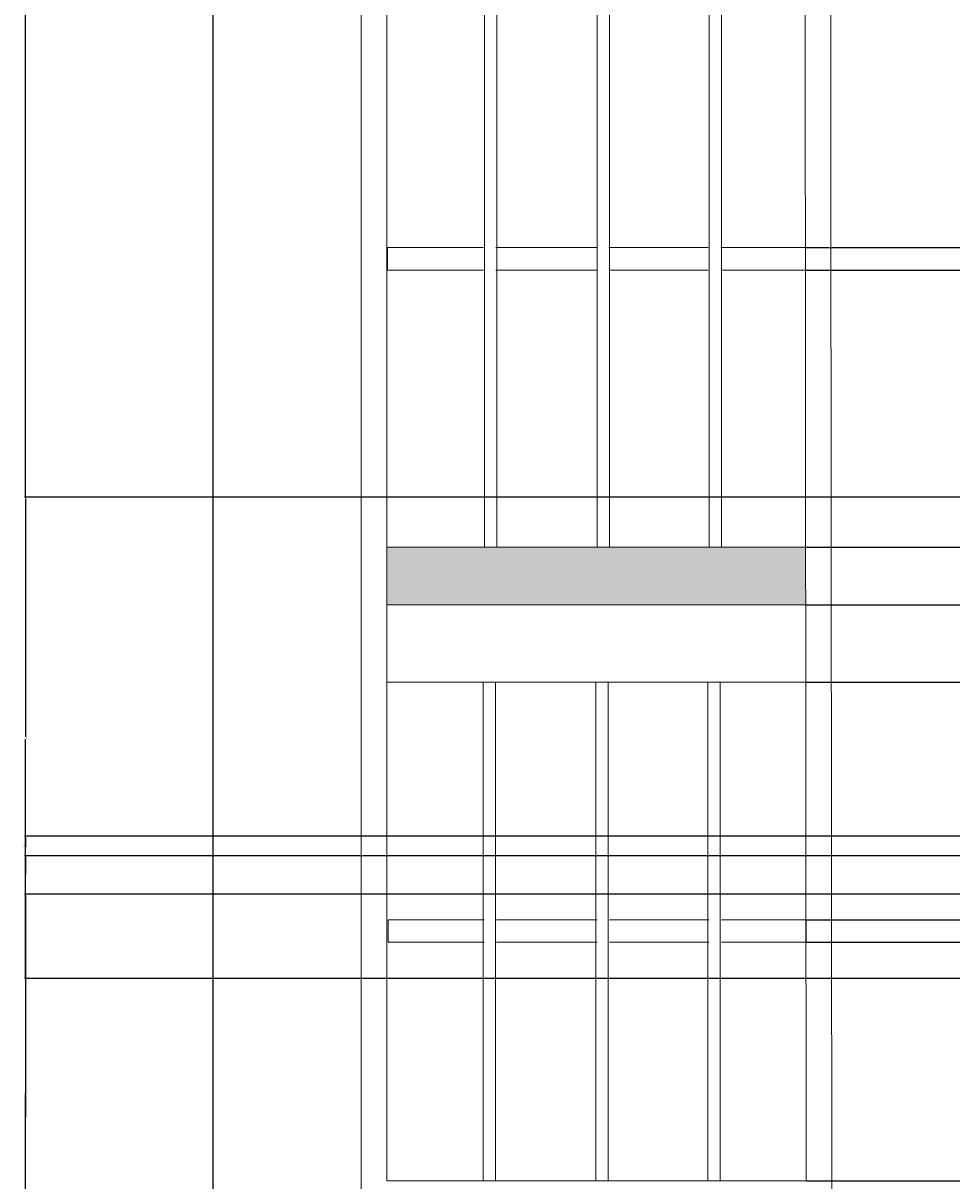
# Model space of a CAD drawing. Units: inches. Extents: x -14 to 375, y -86 to 549.
# Tile 6 of 12: x -14 to 130, y 156 to 336. Entities that reach past the tile are written whole.
import ezdxf

# ---------------------------------------------------------------- set-up
doc = ezdxf.new("R2010")
doc.units = ezdxf.units.IN
doc.header["$MEASUREMENT"] = 0
for name, color, linetype, lineweight in [('A-ANNO-DIMS', 2, 'Continuous', 18), ('A-ELEV', 7, 'Continuous', 25), ('A-ELEV-PATT', 8, 'Continuous', 13), ('A-GLAZ', 4, 'Continuous', 18)]:
    doc.layers.add(name, color=color, linetype=linetype, lineweight=lineweight)
doc.styles.get("Standard").update_dxf_attribs({"font": 'arial.ttf'})
doc.dimstyles.get("Standard").update_dxf_attribs({"dimtxt": 0.18, "dimasz": 0.18, "dimexe": 0.18, "dimexo": 0.0625, "dimgap": 0.09, "dimtad": 0, "dimtih": 1, "dimtoh": 1, "dimdec": 4, "dimzin": 0, "dimdsep": 46, "dimtxsty": 'Standard', "dimcen": 0.09, "dimadec": 0, "dimazin": 0, "dimtfac": 1, "dimtdec": 4, "dimtofl": 0, "dimtmove": 0, "dimatfit": 3, "dimfxl": 1, "dimtolj": 1, "dimtzin": 0, "dimarcsym": 0})

# ---------------------------------------------------------------- blocks, each defined once
blk = doc.blocks.new('*D15')
at = {"layer": 'A-ANNO-DIMS', "color": 0, "lineweight": -2, "transparency": 16777216}
for p, q in [((134.17, 187.85), (-13.88, 187.85)), ((-13.7, 187.67), (-13.7, 170.29)), ((-13.7, 152.56), (-13.7, 169.93)), ((38.44, 152.38), (-13.88, 152.38))]:
    blk.add_line(p, q, dxfattribs=at)
at = {"layer": 'A-ANNO-DIMS', "color": 0, "transparency": 16777216}
for points in [[(-13.73, 187.67), (-13.67, 187.67), (-13.7, 187.85)], [(-13.73, 152.56), (-13.67, 152.56), (-13.7, 152.38)]]:
    blk.add_solid(points, dxfattribs=at)
at = {"layer": 'Defpoints', "color": 0, "transparency": 16777216}
for p in [(-13.7, 187.85), (134.23, 187.85), (38.5, 152.38)]:
    blk.add_point(p, dxfattribs=at)
at = {"layer": 'A-ANNO-DIMS', "color": 0, "transparency": 16777216, "insert": (-13.7, 170.11), "char_height": 0.18, "attachment_point": 5}
blk.add_mtext('\\A1;35.47', dxfattribs=at)
blk = doc.blocks.new('*D16')
at = {"layer": 'A-ANNO-DIMS', "color": 0, "lineweight": -2, "transparency": 16777216}
for p, q in [((134.17, 262.71), (-13.88, 262.71)), ((-13.7, 262.53), (-13.7, 225.46)), ((-13.7, 188.03), (-13.7, 225.09)), ((134.17, 187.85), (-13.88, 187.85))]:
    blk.add_line(p, q, dxfattribs=at)
at = {"layer": 'A-ANNO-DIMS', "color": 0, "transparency": 16777216}
for points in [[(-13.73, 262.53), (-13.67, 262.53), (-13.7, 262.71)], [(-13.73, 188.03), (-13.67, 188.03), (-13.7, 187.85)]]:
    blk.add_solid(points, dxfattribs=at)
at = {"layer": 'Defpoints', "color": 0, "transparency": 16777216}
for p in [(-13.7, 262.71), (134.23, 262.71), (134.23, 187.85)]:
    blk.add_point(p, dxfattribs=at)
at = {"layer": 'A-ANNO-DIMS', "color": 0, "transparency": 16777216, "insert": (-13.7, 225.28), "char_height": 0.18, "attachment_point": 5}
blk.add_mtext('\\A1;74.86', dxfattribs=at)
blk = doc.blocks.new('*D17')
at = {"layer": 'A-ANNO-DIMS', "color": 0, "lineweight": -2, "transparency": 16777216}
for p, q in [((38.44, 432.97), (-13.88, 432.97)), ((-13.7, 432.79), (-13.7, 348.02)), ((-13.7, 262.89), (-13.7, 347.66)), ((134.17, 262.71), (-13.88, 262.71))]:
    blk.add_line(p, q, dxfattribs=at)
at = {"layer": 'A-ANNO-DIMS', "color": 0, "transparency": 16777216}
for points in [[(-13.73, 432.79), (-13.67, 432.79), (-13.7, 432.97)], [(-13.73, 262.89), (-13.67, 262.89), (-13.7, 262.71)]]:
    blk.add_solid(points, dxfattribs=at)
at = {"layer": 'Defpoints', "color": 0, "transparency": 16777216}
for p in [(-13.7, 432.97), (38.5, 432.97), (134.23, 262.71)]:
    blk.add_point(p, dxfattribs=at)
at = {"layer": 'A-ANNO-DIMS', "color": 0, "transparency": 16777216, "insert": (-13.7, 347.84), "char_height": 0.18, "attachment_point": 5}
blk.add_mtext('\\A1;170.26', dxfattribs=at)
blk = doc.blocks.new('*D29')
at = {"layer": 'A-ANNO-DIMS', "color": 0, "lineweight": -2, "transparency": 16777216}
for p, q in [((107.74, 193.48), (374.54, 193.48)), ((374.36, 193.3), (374.36, 175.11)), ((374.36, 156.56), (374.36, 174.75)), ((107.76, 156.38), (374.54, 156.38))]:
    blk.add_line(p, q, dxfattribs=at)
at = {"layer": 'A-ANNO-DIMS', "color": 0, "transparency": 16777216}
for points in [[(374.33, 193.3), (374.39, 193.3), (374.36, 193.48)], [(374.33, 156.56), (374.39, 156.56), (374.36, 156.38)]]:
    blk.add_solid(points, dxfattribs=at)
at = {"layer": 'Defpoints', "color": 0, "transparency": 16777216}
for p in [(107.68, 193.48), (374.36, 193.48), (107.7, 156.38)]:
    blk.add_point(p, dxfattribs=at)
at = {"layer": 'A-ANNO-DIMS', "color": 0, "transparency": 16777216, "insert": (374.36, 174.93), "char_height": 0.18, "attachment_point": 5}
blk.add_mtext('\\A1;37.106', dxfattribs=at)
blk = doc.blocks.new('*D30')
at = {"layer": 'A-ANNO-DIMS', "color": 0, "lineweight": -2, "transparency": 16777216}
for p, q in [((107.74, 196.98), (374.54, 196.98)), ((374.36, 196.8), (374.36, 195.41)), ((374.36, 193.66), (374.36, 195.05)), ((107.74, 193.48), (374.54, 193.48))]:
    blk.add_line(p, q, dxfattribs=at)
at = {"layer": 'A-ANNO-DIMS', "color": 0, "transparency": 16777216}
for points in [[(374.33, 196.8), (374.39, 196.8), (374.36, 196.98)], [(374.33, 193.66), (374.39, 193.66), (374.36, 193.48)]]:
    blk.add_solid(points, dxfattribs=at)
at = {"layer": 'Defpoints', "color": 0, "transparency": 16777216}
for p in [(107.68, 196.98), (374.36, 196.98), (107.68, 193.48)]:
    blk.add_point(p, dxfattribs=at)
at = {"layer": 'A-ANNO-DIMS', "color": 0, "transparency": 16777216, "insert": (374.36, 195.23), "char_height": 0.18, "attachment_point": 5}
blk.add_mtext('\\A1;3.501', dxfattribs=at)
blk = doc.blocks.new('*D31')
at = {"layer": 'A-ANNO-DIMS', "color": 0, "lineweight": -2, "transparency": 16777216}
for p, q in [((107.76, 233.96), (374.54, 233.96)), ((374.36, 233.78), (374.36, 215.65)), ((374.36, 197.16), (374.36, 215.29)), ((107.74, 196.98), (374.54, 196.98))]:
    blk.add_line(p, q, dxfattribs=at)
at = {"layer": 'A-ANNO-DIMS', "color": 0, "transparency": 16777216}
for points in [[(374.33, 233.78), (374.39, 233.78), (374.36, 233.96)], [(374.33, 197.16), (374.39, 197.16), (374.36, 196.98)]]:
    blk.add_solid(points, dxfattribs=at)
at = {"layer": 'Defpoints', "color": 0, "transparency": 16777216}
for p in [(107.7, 233.96), (374.36, 233.96), (107.68, 196.98)]:
    blk.add_point(p, dxfattribs=at)
at = {"layer": 'A-ANNO-DIMS', "color": 0, "transparency": 16777216, "insert": (374.36, 215.47), "char_height": 0.18, "attachment_point": 5}
blk.add_mtext('\\A1;36.975', dxfattribs=at)
blk = doc.blocks.new('*D32')
at = {"layer": 'A-ANNO-DIMS', "color": 0, "lineweight": -2, "transparency": 16777216}
for p, q in [((107.76, 245.96), (374.54, 245.96)), ((374.36, 245.78), (374.36, 240.14)), ((374.36, 234.14), (374.36, 239.78)), ((107.76, 233.96), (374.54, 233.96))]:
    blk.add_line(p, q, dxfattribs=at)
at = {"layer": 'A-ANNO-DIMS', "color": 0, "transparency": 16777216}
for points in [[(374.33, 245.78), (374.39, 245.78), (374.36, 245.96)], [(374.33, 234.14), (374.39, 234.14), (374.36, 233.96)]]:
    blk.add_solid(points, dxfattribs=at)
at = {"layer": 'Defpoints', "color": 0, "transparency": 16777216}
for p in [(107.7, 245.96), (374.36, 245.96), (107.7, 233.96)]:
    blk.add_point(p, dxfattribs=at)
at = {"layer": 'A-ANNO-DIMS', "color": 0, "transparency": 16777216, "insert": (374.36, 239.96), "char_height": 0.18, "attachment_point": 5}
blk.add_mtext('\\A1;12', dxfattribs=at)
blk = doc.blocks.new('*D33')
at = {"layer": 'A-ANNO-DIMS', "color": 0, "lineweight": -2, "transparency": 16777216}
for p, q in [((107.76, 254.96), (374.54, 254.96)), ((374.36, 254.78), (374.36, 250.64)), ((374.36, 246.14), (374.36, 250.28)), ((107.76, 245.96), (374.54, 245.96))]:
    blk.add_line(p, q, dxfattribs=at)
at = {"layer": 'A-ANNO-DIMS', "color": 0, "transparency": 16777216}
for points in [[(374.33, 254.78), (374.39, 254.78), (374.36, 254.96)], [(374.33, 246.14), (374.39, 246.14), (374.36, 245.96)]]:
    blk.add_solid(points, dxfattribs=at)
at = {"layer": 'Defpoints', "color": 0, "transparency": 16777216}
for p in [(107.7, 254.96), (374.36, 254.96), (107.7, 245.96)]:
    blk.add_point(p, dxfattribs=at)
at = {"layer": 'A-ANNO-DIMS', "color": 0, "transparency": 16777216, "insert": (374.36, 250.46), "char_height": 0.18, "attachment_point": 5}
blk.add_mtext('\\A1;9', dxfattribs=at)
blk = doc.blocks.new('*D34')
at = {"layer": 'A-ANNO-DIMS', "color": 0, "lineweight": -2, "transparency": 16777216}
for p, q in [((107.64, 298.04), (374.54, 298.04)), ((374.36, 297.86), (374.36, 276.68)), ((374.36, 255.14), (374.36, 276.32)), ((107.76, 254.96), (374.54, 254.96))]:
    blk.add_line(p, q, dxfattribs=at)
at = {"layer": 'A-ANNO-DIMS', "color": 0, "transparency": 16777216}
for points in [[(374.33, 297.86), (374.39, 297.86), (374.36, 298.04)], [(374.33, 255.14), (374.39, 255.14), (374.36, 254.96)]]:
    blk.add_solid(points, dxfattribs=at)
at = {"layer": 'Defpoints', "color": 0, "transparency": 16777216}
for p in [(107.58, 298.04), (374.36, 298.04), (107.7, 254.96)]:
    blk.add_point(p, dxfattribs=at)
at = {"layer": 'A-ANNO-DIMS', "color": 0, "transparency": 16777216, "insert": (374.36, 276.5), "char_height": 0.18, "attachment_point": 5}
blk.add_mtext('\\A1;43.08', dxfattribs=at)
blk = doc.blocks.new('*D35')
at = {"layer": 'A-ANNO-DIMS', "color": 0, "lineweight": -2, "transparency": 16777216}
for p, q in [((107.64, 301.54), (374.54, 301.54)), ((374.36, 301.36), (374.36, 299.97)), ((374.36, 298.22), (374.36, 299.6)), ((107.64, 298.04), (374.54, 298.04))]:
    blk.add_line(p, q, dxfattribs=at)
at = {"layer": 'A-ANNO-DIMS', "color": 0, "transparency": 16777216}
for points in [[(374.33, 301.36), (374.39, 301.36), (374.36, 301.54)], [(374.33, 298.22), (374.39, 298.22), (374.36, 298.04)]]:
    blk.add_solid(points, dxfattribs=at)
at = {"layer": 'Defpoints', "color": 0, "transparency": 16777216}
for p in [(107.58, 301.54), (374.36, 301.54), (107.58, 298.04)]:
    blk.add_point(p, dxfattribs=at)
at = {"layer": 'A-ANNO-DIMS', "color": 0, "transparency": 16777216, "insert": (374.36, 299.79), "char_height": 0.18, "attachment_point": 5}
blk.add_mtext('\\A1;3.501', dxfattribs=at)
blk = doc.blocks.new('*D36')
at = {"layer": 'A-ANNO-DIMS', "color": 0, "lineweight": -2, "transparency": 16777216}
for p, q in [((107.56, 353.96), (374.54, 353.96)), ((374.36, 353.78), (374.36, 327.93)), ((374.36, 301.72), (374.36, 327.57)), ((107.64, 301.54), (374.54, 301.54))]:
    blk.add_line(p, q, dxfattribs=at)
at = {"layer": 'A-ANNO-DIMS', "color": 0, "transparency": 16777216}
for points in [[(374.33, 353.78), (374.39, 353.78), (374.36, 353.96)], [(374.33, 301.72), (374.39, 301.72), (374.36, 301.54)]]:
    blk.add_solid(points, dxfattribs=at)
at = {"layer": 'Defpoints', "color": 0, "transparency": 16777216}
for p in [(107.5, 353.96), (374.36, 353.96), (107.58, 301.54)]:
    blk.add_point(p, dxfattribs=at)
at = {"layer": 'A-ANNO-DIMS', "color": 0, "transparency": 16777216, "insert": (374.36, 327.75), "char_height": 0.18, "attachment_point": 5}
blk.add_mtext('\\A1;52.42', dxfattribs=at)
blk = doc.blocks.new('*D96')
at = {"layer": 'A-ANNO-DIMS', "color": 0, "lineweight": -2, "transparency": 16777216}
for p, q in [((194.3, 200.95), (-13.88, 200.95)), ((-13.7, 200.77), (-13.7, 166.64)), ((-13.7, 132.15), (-13.7, 166.28)), ((194.3, 131.97), (-13.88, 131.97))]:
    blk.add_line(p, q, dxfattribs=at)
at = {"layer": 'A-ANNO-DIMS', "color": 0, "transparency": 16777216}
for points in [[(-13.73, 200.77), (-13.67, 200.77), (-13.7, 200.95)], [(-13.73, 132.15), (-13.67, 132.15), (-13.7, 131.97)]]:
    blk.add_solid(points, dxfattribs=at)
at = {"layer": 'Defpoints', "color": 0, "transparency": 16777216}
for p in [(-13.7, 200.95), (194.37, 200.95), (194.37, 131.97)]:
    blk.add_point(p, dxfattribs=at)
at = {"layer": 'A-ANNO-DIMS', "color": 0, "transparency": 16777216, "insert": (-13.7, 166.46), "char_height": 0.18, "attachment_point": 5}
blk.add_mtext('\\A1;68.98', dxfattribs=at)
blk = doc.blocks.new('*D97')
at = {"layer": 'A-ANNO-DIMS', "color": 0, "lineweight": -2, "transparency": 16777216}
for p, q in [((190.3, 206.95), (-13.88, 206.95)), ((-13.7, 206.77), (-13.7, 204.13)), ((-13.7, 201.13), (-13.7, 203.77)), ((194.3, 200.95), (-13.88, 200.95))]:
    blk.add_line(p, q, dxfattribs=at)
at = {"layer": 'A-ANNO-DIMS', "color": 0, "transparency": 16777216}
for points in [[(-13.73, 206.77), (-13.67, 206.77), (-13.7, 206.95)], [(-13.73, 201.13), (-13.67, 201.13), (-13.7, 200.95)]]:
    blk.add_solid(points, dxfattribs=at)
at = {"layer": 'Defpoints', "color": 0, "transparency": 16777216}
for p in [(-13.7, 206.95), (190.37, 206.95), (194.37, 200.95)]:
    blk.add_point(p, dxfattribs=at)
at = {"layer": 'A-ANNO-DIMS', "color": 0, "transparency": 16777216, "insert": (-13.7, 203.95), "char_height": 0.18, "attachment_point": 5}
blk.add_mtext('\\A1;6', dxfattribs=at)
blk = doc.blocks.new('*D98')
at = {"layer": 'A-ANNO-DIMS', "color": 0, "lineweight": -2, "transparency": 16777216}
for p, q in [((187.3, 209.97), (-13.88, 209.97)), ((-13.7, 209.79), (-13.7, 208.64)), ((-13.7, 207.13), (-13.7, 208.28)), ((190.3, 206.95), (-13.88, 206.95))]:
    blk.add_line(p, q, dxfattribs=at)
at = {"layer": 'A-ANNO-DIMS', "color": 0, "transparency": 16777216}
for points in [[(-13.73, 209.79), (-13.67, 209.79), (-13.7, 209.97)], [(-13.73, 207.13), (-13.67, 207.13), (-13.7, 206.95)]]:
    blk.add_solid(points, dxfattribs=at)
at = {"layer": 'Defpoints', "color": 0, "transparency": 16777216}
for p in [(-13.7, 209.97), (187.37, 209.97), (190.37, 206.95)]:
    blk.add_point(p, dxfattribs=at)
at = {"layer": 'A-ANNO-DIMS', "color": 0, "transparency": 16777216, "insert": (-13.7, 208.46), "char_height": 0.18, "attachment_point": 5}
blk.add_mtext('\\A1;3.023', dxfattribs=at)

msp = doc.modelspace()

# ---------------------------------------------------------------- hatches: boundary and pattern name
at = {"layer": 'A-ELEV-PATT'}
h = msp.add_hatch(dxfattribs=at)
h.set_pattern_fill('SWAMP', color=256, scale=0.8)
h.set_pattern_definition([(0, (-168.40604, -22.7026), (0.4, 0.6928203), [0.1, -0.7]), (90, (-168.35604, -22.7026), (-0.4, 0.69282032), [0.05, -1.3356406]), (90, (-168.34354, -22.7026), (-0.4, 0.69282032), [0.04, -1.3456406]), (90, (-168.36854, -22.7026), (-0.4, 0.69282032), [0.04, -1.3456406]), (60, (-168.33104, -22.7026), (-0.4, 0.6928203), [0.032, -0.768]), (120, (-168.38104, -22.7026), (-0.8, 3e-10), [0.032, -0.768])])
h.paths.add_polyline_path([(42.5033, 374.9589), (42.5033, 365.9589), (107.4987, 365.9589), (107.4987, 374.9589)])
h.paths.add_polyline_path([(107.615, 245.9589), (107.6063, 254.9589), (42.5033, 254.9589), (42.5033, 245.9589)])

# ---------------------------------------------------------------- linework, layer by layer
at = {"layer": 'A-ELEV'}
for p, q in [((15.4018, 365.9589), (15.4018, 245.9589)), ((15.4018, 245.9589), (15.4018, 125.9589))]:
    msp.add_line(p, q, dxfattribs=at)
at = {"layer": 'A-GLAZ'}
for p, q in [((107.4899, 374.9589), (107.7019, 156.3768)), ((57.6445, 254.9589), (57.6445, 353.9589)), ((59.5668, 353.9589), (59.5668, 254.9589)), ((75.2042, 254.9589), (75.2042, 353.9589)), ((77.1265, 353.9589), (77.1265, 254.9589)), ((92.5999, 254.9589), (92.5999, 353.9589)), ((94.5222, 353.9589), (94.5222, 254.9589)), ((42.5033, 254.9589), (107.7019, 254.9589)), ((59.5668, 254.9589), (57.6445, 254.9589)), ((77.1265, 254.9589), (75.2042, 254.9589)), ((94.5222, 254.9589), (92.5999, 254.9589)), ((42.5033, 245.9589), (107.7019, 245.9589)), ((107.7019, 245.9589), (42.5033, 245.9589)), ((42.5033, 233.9589), (107.7019, 233.9589)), ((107.7019, 156.3768), (42.5033, 156.3768))]:
    msp.add_line(p, q, dxfattribs=at)
for points in [[(111.4987, 365.9589), (111.7019, 152.3768), (38.5033, 152.3768), (38.5033, 365.9589), (38.5033, 432.9679, -0.90920588), (111.4987, 432.9679), (111.4987, 365.9589)], [(42.5033, 156.3768), (42.5033, 365.9589), (42.5033, 432.7722, -0.9040533), (107.4987, 432.7722), (107.4987, 365.9589)]]:
    msp.add_lwpolyline(points, format="xyb", dxfattribs=at)
for points in [[(57.521, 301.5363), (42.5831, 301.5363), (42.5831, 298.0352), (57.521, 298.0352)], [(75.0807, 301.5363), (59.4433, 301.5363)], [(92.4765, 301.5363), (77.003, 301.5363)], [(94.3987, 298.0352), (107.5784, 298.0352), (107.5784, 301.5363), (94.3987, 301.5363)], [(59.4433, 298.0352), (75.0807, 298.0352)], [(77.003, 298.0352), (92.4765, 298.0352)], [(59.3636, 233.9589), (59.3636, 156.3768), (57.4413, 156.3768), (57.4413, 233.9589)], [(76.9233, 233.9589), (76.9233, 156.3768), (75.001, 156.3768), (75.001, 233.9589)], [(94.319, 233.9589), (94.319, 156.3768), (92.3967, 156.3768), (92.3967, 233.9589)], [(57.6224, 196.9836), (42.6844, 196.9836), (42.6844, 193.4825), (57.6224, 193.4825)], [(75.1821, 196.9836), (59.5447, 196.9836)], [(92.5778, 196.9836), (77.1044, 196.9836)], [(94.5001, 193.4825), (107.6798, 193.4825), (107.6798, 196.9836), (94.5001, 196.9836)], [(59.5447, 193.4825), (75.1821, 193.4825)], [(77.1044, 193.4825), (92.5778, 193.4825)]]:
    msp.add_lwpolyline(points, dxfattribs=at)

# ---------------------------------------------------------------- dimensions: what is measured, and where the dimension line sits
at = {"layer": 'A-ANNO-DIMS'}
for base, p1, p2, override, picture, middle in [((-13.6982, 432.9679), (134.2334, 262.7071), (38.5033, 432.9679), {"dimdec": 2, "dimlfac": 1, "dimrnd": 0, "dimzin": 0, "dimdsep": 46, "dimlunit": 2}, '*D17', (-13.6982, 347.8375)), ((374.3647, 353.9589), (107.5784, 301.5363), (107.4987, 353.9589), {"dimdec": 2, "dimlfac": 1, "dimrnd": 0, "dimzin": 0, "dimdsep": 46, "dimlunit": 2}, '*D36', (374.3647, 327.7476)), ((374.3647, 301.5363), (107.5784, 298.0352), (107.5784, 301.5363), {"dimdec": 3, "dimlfac": 1, "dimrnd": 0, "dimzin": 0, "dimdsep": 46, "dimlunit": 2}, '*D35', (374.3647, 299.7857)), ((374.3647, 298.0352), (107.7019, 254.9589), (107.5784, 298.0352), {"dimdec": 2, "dimlfac": 1, "dimrnd": 0, "dimzin": 0, "dimdsep": 46, "dimlunit": 2}, '*D34', (374.3647, 276.4971)), ((-13.6982, 262.7071), (134.2334, 187.8466), (134.2334, 262.7071), {"dimdec": 2, "dimlfac": 1, "dimrnd": 0, "dimzin": 0, "dimdsep": 46, "dimlunit": 2}, '*D16', (-13.6982, 225.2768)), ((374.3647, 254.9589), (107.7019, 245.9589), (107.7019, 254.9589), {"dimdec": 0, "dimlfac": 1, "dimrnd": 0, "dimzin": 0, "dimdsep": 46, "dimlunit": 2}, '*D33', (374.3647, 250.4589)), ((374.3647, 245.9589), (107.7019, 233.9589), (107.7019, 245.9589), {"dimdec": 0, "dimlfac": 1, "dimrnd": 0, "dimzin": 0, "dimdsep": 46, "dimlunit": 2}, '*D32', (374.3647, 239.9589)), ((374.3647, 233.9589), (107.6798, 196.9836), (107.7019, 233.9589), {"dimdec": 3, "dimlfac": 1, "dimrnd": 0, "dimzin": 0, "dimdsep": 46, "dimlunit": 2}, '*D31', (374.3647, 215.4712)), ((-13.6982, 209.9717), (190.3657, 206.9487), (187.3657, 209.9717), {"dimdec": 3, "dimlfac": 1, "dimrnd": 0, "dimzin": 0, "dimdsep": 46, "dimlunit": 2}, '*D98', (-13.6982, 208.4602)), ((-13.6982, 206.9487), (194.3657, 200.9487), (190.3657, 206.9487), {"dimdec": 0, "dimlfac": 1, "dimrnd": 0, "dimzin": 0, "dimdsep": 46, "dimlunit": 2}, '*D97', (-13.6982, 203.9487)), ((-13.6982, 200.9487), (194.3657, 131.9717), (194.3657, 200.9487), {"dimdec": 2, "dimlfac": 1, "dimrnd": 0, "dimzin": 0, "dimdsep": 46, "dimlunit": 2}, '*D96', (-13.6982, 166.4602)), ((374.3647, 196.9836), (107.6798, 193.4825), (107.6798, 196.9836), {"dimdec": 3, "dimlfac": 1, "dimrnd": 0, "dimzin": 0, "dimdsep": 46, "dimlunit": 2}, '*D30', (374.3647, 195.233)), ((374.3647, 193.4825), (107.7019, 156.3768), (107.6798, 193.4825), {"dimdec": 3, "dimlfac": 1, "dimrnd": 0, "dimzin": 0, "dimdsep": 46, "dimlunit": 2}, '*D29', (374.3647, 174.9296)), ((-13.6982, 187.8466), (38.5033, 152.3768), (134.2334, 187.8466), {"dimdec": 2, "dimlfac": 1, "dimrnd": 0, "dimzin": 0, "dimdsep": 46, "dimlunit": 2}, '*D15', (-13.6982, 170.1117))]:
    dim = msp.add_linear_dim(base=base, p1=p1, p2=p2, angle=90, dimstyle='Standard', override=override, dxfattribs=at)
    dim.commit()
    dim.dimension.update_dxf_attribs({"geometry": picture, "text_midpoint": middle})

doc.saveas('drawing.dxf')
